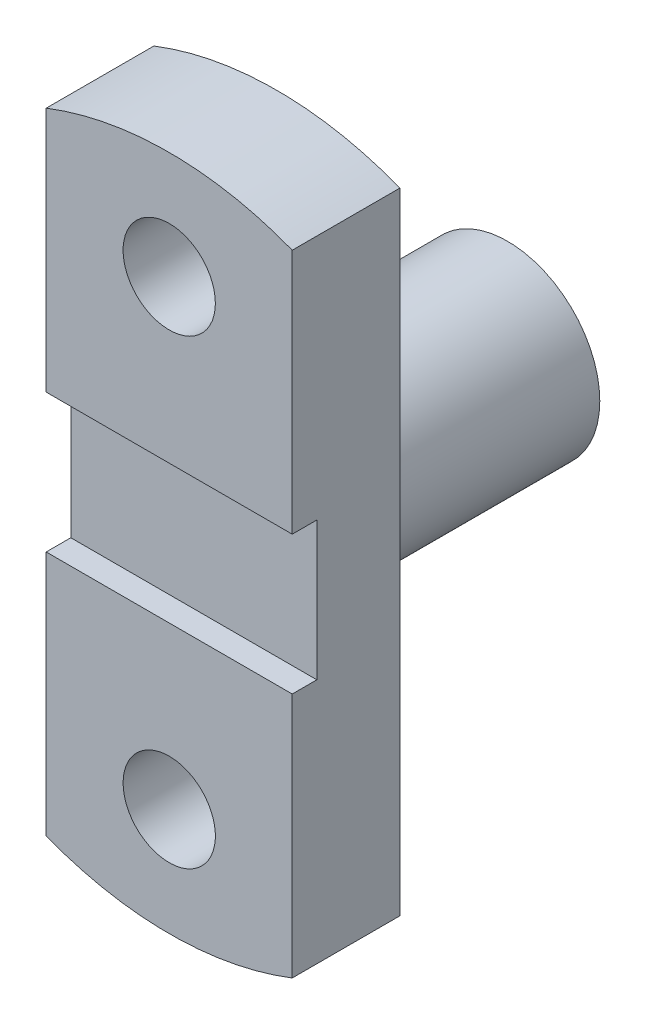
ISO-10303-21;
HEADER;
FILE_DESCRIPTION(('STEP AP214'),'2;1');
FILE_NAME('part.step','',(''),(''),'','','');
FILE_SCHEMA(('AUTOMOTIVE_DESIGN { 1 0 10303 214 1 1 1 1 }'));
ENDSEC;
DATA;
#1=APPLICATION_CONTEXT('core data for automotive mechanical design processes');
#2=APPLICATION_PROTOCOL_DEFINITION('international standard','automotive_design',2000,#1);
#3=PRODUCT_CONTEXT('',#1,'mechanical');
#4=PRODUCT('Part','Part','',(#3));
#5=PRODUCT_RELATED_PRODUCT_CATEGORY('part','',(#4));
#6=PRODUCT_DEFINITION_FORMATION('','',#4);
#7=PRODUCT_DEFINITION_CONTEXT('part definition',#1,'design');
#8=PRODUCT_DEFINITION('design','',#6,#7);
#9=PRODUCT_DEFINITION_SHAPE('','',#8);
#10=(LENGTH_UNIT() NAMED_UNIT(*) SI_UNIT(.MILLI.,.METRE.));
#11=(NAMED_UNIT(*) PLANE_ANGLE_UNIT() SI_UNIT($,.RADIAN.));
#12=(NAMED_UNIT(*) SI_UNIT($,.STERADIAN.) SOLID_ANGLE_UNIT());
#13=UNCERTAINTY_MEASURE_WITH_UNIT(LENGTH_MEASURE(1.E-05),#10,'distance_accuracy_value','');
#14=(GEOMETRIC_REPRESENTATION_CONTEXT(3) GLOBAL_UNCERTAINTY_ASSIGNED_CONTEXT((#13)) GLOBAL_UNIT_ASSIGNED_CONTEXT((#10,
#11,#12)) REPRESENTATION_CONTEXT('',''));
#15=CARTESIAN_POINT('',(0.,0.,0.));
#16=DIRECTION('',(0.,0.,1.));
#17=DIRECTION('',(1.,0.,0.));
#18=AXIS2_PLACEMENT_3D('',#15,#16,#17);
#19=CARTESIAN_POINT('',(0.,0.,17.5));
#20=DIRECTION('',(0.,0.,-1.));
#21=DIRECTION('',(-1.,0.,0.));
#22=AXIS2_PLACEMENT_3D('',#19,#20,#21);
#23=PLANE('',#22);
#24=CARTESIAN_POINT('',(0.,75.,17.5));
#25=DIRECTION('',(0.,0.,1.));
#26=DIRECTION('',(1.,0.,0.));
#27=AXIS2_PLACEMENT_3D('',#24,#25,#26);
#28=CIRCLE('',#27,15.);
#29=CARTESIAN_POINT('',(15.,75.,17.5));
#30=VERTEX_POINT('',#29);
#31=EDGE_CURVE('E153',#30,#30,#28,.T.);
#32=ORIENTED_EDGE('',*,*,#31,.F.);
#33=EDGE_LOOP('',(#32));
#34=FACE_BOUND('',#33,.T.);
#35=DIRECTION('',(0.,-1.,0.));
#36=VECTOR('',#35,1.);
#37=CARTESIAN_POINT('',(-40.,-102.469507659596,17.5));
#38=LINE('',#37,#36);
#39=CARTESIAN_POINT('',(-40.,102.469507659596,17.5));
#40=VERTEX_POINT('',#39);
#41=CARTESIAN_POINT('',(-40.,22.5,17.5));
#42=VERTEX_POINT('',#41);
#43=EDGE_CURVE('E95',#40,#42,#38,.T.);
#44=ORIENTED_EDGE('',*,*,#43,.T.);
#45=DIRECTION('',(1.,0.,0.));
#46=VECTOR('',#45,1.);
#47=CARTESIAN_POINT('',(-85.7055795281058,22.5,17.5));
#48=LINE('',#47,#46);
#49=CARTESIAN_POINT('',(40.,22.5,17.5));
#50=VERTEX_POINT('',#49);
#51=EDGE_CURVE('E136',#42,#50,#48,.T.);
#52=ORIENTED_EDGE('',*,*,#51,.T.);
#53=DIRECTION('',(0.,1.,0.));
#54=VECTOR('',#53,1.);
#55=CARTESIAN_POINT('',(40.,-102.469507659596,17.5));
#56=LINE('',#55,#54);
#57=CARTESIAN_POINT('',(40.,102.469507659596,17.5));
#58=VERTEX_POINT('',#57);
#59=EDGE_CURVE('E62',#50,#58,#56,.T.);
#60=ORIENTED_EDGE('',*,*,#59,.T.);
#61=CARTESIAN_POINT('',(0.,0.,17.5));
#62=DIRECTION('',(0.,0.,1.));
#63=DIRECTION('',(-1.,0.,0.));
#64=AXIS2_PLACEMENT_3D('',#61,#62,#63);
#65=CIRCLE('',#64,110.);
#66=EDGE_CURVE('E157',#58,#40,#65,.T.);
#67=ORIENTED_EDGE('',*,*,#66,.T.);
#68=EDGE_LOOP('',(#44,#52,#60,#67));
#69=FACE_BOUND('',#68,.T.);
#70=ADVANCED_FACE('F39',(#34,#69),#23,.F.);
#71=CARTESIAN_POINT('',(40.,-102.469507659596,17.5));
#72=VERTEX_POINT('',#71);
#73=CARTESIAN_POINT('',(40.,-22.5,17.5));
#74=VERTEX_POINT('',#73);
#75=EDGE_CURVE('E164',#72,#74,#56,.T.);
#76=ORIENTED_EDGE('',*,*,#75,.T.);
#77=DIRECTION('',(1.,0.,0.));
#78=VECTOR('',#77,1.);
#79=CARTESIAN_POINT('',(-85.7055795281058,-22.5,17.5));
#80=LINE('',#79,#78);
#81=CARTESIAN_POINT('',(-40.,-22.5,17.5));
#82=VERTEX_POINT('',#81);
#83=EDGE_CURVE('E53',#82,#74,#80,.T.);
#84=ORIENTED_EDGE('',*,*,#83,.F.);
#85=CARTESIAN_POINT('',(-40.,-102.469507659596,17.5));
#86=VERTEX_POINT('',#85);
#87=EDGE_CURVE('E161',#82,#86,#38,.T.);
#88=ORIENTED_EDGE('',*,*,#87,.T.);
#89=CARTESIAN_POINT('',(0.,0.,17.5));
#90=DIRECTION('',(0.,0.,1.));
#91=DIRECTION('',(1.,0.,0.));
#92=AXIS2_PLACEMENT_3D('',#89,#90,#91);
#93=CIRCLE('',#92,110.);
#94=EDGE_CURVE('E162',#86,#72,#93,.T.);
#95=ORIENTED_EDGE('',*,*,#94,.T.);
#96=EDGE_LOOP('',(#76,#84,#88,#95));
#97=FACE_BOUND('',#96,.T.);
#98=CARTESIAN_POINT('',(0.,-74.9999999999999,17.5));
#99=DIRECTION('',(0.,0.,1.));
#100=DIRECTION('',(-1.,0.,0.));
#101=AXIS2_PLACEMENT_3D('',#98,#99,#100);
#102=CIRCLE('',#101,15.);
#103=CARTESIAN_POINT('',(-15.,-74.9999999999999,17.5));
#104=VERTEX_POINT('',#103);
#105=EDGE_CURVE('E150',#104,#104,#102,.T.);
#106=ORIENTED_EDGE('',*,*,#105,.F.);
#107=EDGE_LOOP('',(#106));
#108=FACE_BOUND('',#107,.T.);
#109=ADVANCED_FACE('F213',(#97,#108),#23,.F.);
#110=CARTESIAN_POINT('',(0.,0.,-17.5));
#111=DIRECTION('',(0.,0.,-1.));
#112=DIRECTION('',(-1.,0.,0.));
#113=AXIS2_PLACEMENT_3D('',#110,#111,#112);
#114=PLANE('',#113);
#115=CARTESIAN_POINT('',(0.,0.,-17.5));
#116=DIRECTION('',(0.,0.,-1.));
#117=DIRECTION('',(-1.,0.,0.));
#118=AXIS2_PLACEMENT_3D('',#115,#116,#117);
#119=CIRCLE('',#118,30.);
#120=CARTESIAN_POINT('',(-30.,0.,-17.5));
#121=VERTEX_POINT('',#120);
#122=EDGE_CURVE('E197',#121,#121,#119,.T.);
#123=ORIENTED_EDGE('',*,*,#122,.F.);
#124=EDGE_LOOP('',(#123));
#125=FACE_BOUND('',#124,.T.);
#126=CARTESIAN_POINT('',(0.,75.,-17.5));
#127=DIRECTION('',(0.,0.,1.));
#128=DIRECTION('',(1.,0.,0.));
#129=AXIS2_PLACEMENT_3D('',#126,#127,#128);
#130=CIRCLE('',#129,15.);
#131=CARTESIAN_POINT('',(15.,75.,-17.5));
#132=VERTEX_POINT('',#131);
#133=EDGE_CURVE('E147',#132,#132,#130,.T.);
#134=ORIENTED_EDGE('',*,*,#133,.T.);
#135=EDGE_LOOP('',(#134));
#136=FACE_BOUND('',#135,.T.);
#137=CARTESIAN_POINT('',(0.,0.,-17.5));
#138=DIRECTION('',(0.,0.,1.));
#139=DIRECTION('',(-1.,0.,0.));
#140=AXIS2_PLACEMENT_3D('',#137,#138,#139);
#141=CIRCLE('',#140,110.);
#142=CARTESIAN_POINT('',(40.,102.469507659596,-17.5));
#143=VERTEX_POINT('',#142);
#144=CARTESIAN_POINT('',(-40.,102.469507659596,-17.5));
#145=VERTEX_POINT('',#144);
#146=EDGE_CURVE('E156',#143,#145,#141,.T.);
#147=ORIENTED_EDGE('',*,*,#146,.F.);
#148=DIRECTION('',(0.,1.,0.));
#149=VECTOR('',#148,1.);
#150=CARTESIAN_POINT('',(40.,-102.469507659596,-17.5));
#151=LINE('',#150,#149);
#152=CARTESIAN_POINT('',(40.,-102.469507659596,-17.5));
#153=VERTEX_POINT('',#152);
#154=EDGE_CURVE('E83',#153,#143,#151,.T.);
#155=ORIENTED_EDGE('',*,*,#154,.F.);
#156=CARTESIAN_POINT('',(0.,0.,-17.5));
#157=DIRECTION('',(0.,0.,1.));
#158=DIRECTION('',(1.,0.,0.));
#159=AXIS2_PLACEMENT_3D('',#156,#157,#158);
#160=CIRCLE('',#159,110.);
#161=CARTESIAN_POINT('',(-40.,-102.469507659596,-17.5));
#162=VERTEX_POINT('',#161);
#163=EDGE_CURVE('E175',#162,#153,#160,.T.);
#164=ORIENTED_EDGE('',*,*,#163,.F.);
#165=DIRECTION('',(0.,-1.,0.));
#166=VECTOR('',#165,1.);
#167=CARTESIAN_POINT('',(-40.,-102.469507659596,-17.5));
#168=LINE('',#167,#166);
#169=EDGE_CURVE('E168',#145,#162,#168,.T.);
#170=ORIENTED_EDGE('',*,*,#169,.F.);
#171=EDGE_LOOP('',(#147,#155,#164,#170));
#172=FACE_BOUND('',#171,.T.);
#173=CARTESIAN_POINT('',(0.,-74.9999999999999,-17.5));
#174=DIRECTION('',(0.,0.,1.));
#175=DIRECTION('',(-1.,0.,0.));
#176=AXIS2_PLACEMENT_3D('',#173,#174,#175);
#177=CIRCLE('',#176,15.);
#178=CARTESIAN_POINT('',(-15.,-74.9999999999999,-17.5));
#179=VERTEX_POINT('',#178);
#180=EDGE_CURVE('E144',#179,#179,#177,.T.);
#181=ORIENTED_EDGE('',*,*,#180,.T.);
#182=EDGE_LOOP('',(#181));
#183=FACE_BOUND('',#182,.T.);
#184=ADVANCED_FACE('F190',(#125,#136,#172,#183),#114,.T.);
#185=CARTESIAN_POINT('',(0.,0.,17.5));
#186=DIRECTION('',(0.,0.,-1.));
#187=DIRECTION('',(-1.,0.,0.));
#188=AXIS2_PLACEMENT_3D('',#185,#186,#187);
#189=CYLINDRICAL_SURFACE('',#188,110.);
#190=ORIENTED_EDGE('',*,*,#146,.T.);
#191=DIRECTION('',(0.,0.,-1.));
#192=VECTOR('',#191,1.);
#193=CARTESIAN_POINT('',(-40.,102.469507659596,17.5));
#194=LINE('',#193,#192);
#195=EDGE_CURVE('E11',#40,#145,#194,.T.);
#196=ORIENTED_EDGE('',*,*,#195,.F.);
#197=ORIENTED_EDGE('',*,*,#66,.F.);
#198=DIRECTION('',(0.,0.,-1.));
#199=VECTOR('',#198,1.);
#200=CARTESIAN_POINT('',(40.,102.469507659596,17.5));
#201=LINE('',#200,#199);
#202=EDGE_CURVE('E170',#58,#143,#201,.T.);
#203=ORIENTED_EDGE('',*,*,#202,.T.);
#204=EDGE_LOOP('',(#190,#196,#197,#203));
#205=FACE_BOUND('',#204,.T.);
#206=ADVANCED_FACE('F41',(#205),#189,.T.);
#207=CARTESIAN_POINT('',(-40.,-102.469507659596,17.5));
#208=DIRECTION('',(1.,0.,0.));
#209=DIRECTION('',(0.,0.,-1.));
#210=AXIS2_PLACEMENT_3D('',#207,#208,#209);
#211=PLANE('',#210);
#212=DIRECTION('',(0.,-1.,0.));
#213=VECTOR('',#212,1.);
#214=CARTESIAN_POINT('',(-40.,22.5,9.5));
#215=LINE('',#214,#213);
#216=CARTESIAN_POINT('',(-40.,22.5,9.5));
#217=VERTEX_POINT('',#216);
#218=CARTESIAN_POINT('',(-40.,-22.5,9.5));
#219=VERTEX_POINT('',#218);
#220=EDGE_CURVE('E124',#217,#219,#215,.T.);
#221=ORIENTED_EDGE('',*,*,#220,.F.);
#222=DIRECTION('',(0.,0.,-1.));
#223=VECTOR('',#222,1.);
#224=CARTESIAN_POINT('',(-40.,22.5,17.5));
#225=LINE('',#224,#223);
#226=EDGE_CURVE('E148',#42,#217,#225,.T.);
#227=ORIENTED_EDGE('',*,*,#226,.F.);
#228=ORIENTED_EDGE('',*,*,#43,.F.);
#229=ORIENTED_EDGE('',*,*,#195,.T.);
#230=ORIENTED_EDGE('',*,*,#169,.T.);
#231=DIRECTION('',(0.,0.,-1.));
#232=VECTOR('',#231,1.);
#233=CARTESIAN_POINT('',(-40.,-102.469507659596,17.5));
#234=LINE('',#233,#232);
#235=EDGE_CURVE('E50',#86,#162,#234,.T.);
#236=ORIENTED_EDGE('',*,*,#235,.F.);
#237=ORIENTED_EDGE('',*,*,#87,.F.);
#238=DIRECTION('',(0.,0.,1.));
#239=VECTOR('',#238,1.);
#240=CARTESIAN_POINT('',(-40.,-22.5,9.5));
#241=LINE('',#240,#239);
#242=EDGE_CURVE('E141',#219,#82,#241,.T.);
#243=ORIENTED_EDGE('',*,*,#242,.F.);
#244=EDGE_LOOP('',(#221,#227,#228,#229,#230,#236,#237,#243));
#245=FACE_BOUND('',#244,.T.);
#246=ADVANCED_FACE('F191',(#245),#211,.F.);
#247=CARTESIAN_POINT('',(0.,0.,17.5));
#248=DIRECTION('',(0.,0.,-1.));
#249=DIRECTION('',(-1.,0.,0.));
#250=AXIS2_PLACEMENT_3D('',#247,#248,#249);
#251=CYLINDRICAL_SURFACE('',#250,110.);
#252=ORIENTED_EDGE('',*,*,#163,.T.);
#253=DIRECTION('',(0.,0.,-1.));
#254=VECTOR('',#253,1.);
#255=CARTESIAN_POINT('',(40.,-102.469507659596,17.5));
#256=LINE('',#255,#254);
#257=EDGE_CURVE('E177',#72,#153,#256,.T.);
#258=ORIENTED_EDGE('',*,*,#257,.F.);
#259=ORIENTED_EDGE('',*,*,#94,.F.);
#260=ORIENTED_EDGE('',*,*,#235,.T.);
#261=EDGE_LOOP('',(#252,#258,#259,#260));
#262=FACE_BOUND('',#261,.T.);
#263=ADVANCED_FACE('F185',(#262),#251,.T.);
#264=CARTESIAN_POINT('',(40.,-102.469507659596,17.5));
#265=DIRECTION('',(-1.,0.,0.));
#266=DIRECTION('',(0.,0.,1.));
#267=AXIS2_PLACEMENT_3D('',#264,#265,#266);
#268=PLANE('',#267);
#269=ORIENTED_EDGE('',*,*,#59,.F.);
#270=DIRECTION('',(0.,0.,1.));
#271=VECTOR('',#270,1.);
#272=CARTESIAN_POINT('',(40.,22.5,17.5));
#273=LINE('',#272,#271);
#274=CARTESIAN_POINT('',(40.,22.5,9.5));
#275=VERTEX_POINT('',#274);
#276=EDGE_CURVE('E133',#275,#50,#273,.T.);
#277=ORIENTED_EDGE('',*,*,#276,.F.);
#278=DIRECTION('',(0.,1.,0.));
#279=VECTOR('',#278,1.);
#280=CARTESIAN_POINT('',(40.,22.5,9.5));
#281=LINE('',#280,#279);
#282=CARTESIAN_POINT('',(40.,-22.5,9.5));
#283=VERTEX_POINT('',#282);
#284=EDGE_CURVE('E119',#283,#275,#281,.T.);
#285=ORIENTED_EDGE('',*,*,#284,.F.);
#286=DIRECTION('',(0.,0.,-1.));
#287=VECTOR('',#286,1.);
#288=CARTESIAN_POINT('',(40.,-22.5,9.5));
#289=LINE('',#288,#287);
#290=EDGE_CURVE('E130',#74,#283,#289,.T.);
#291=ORIENTED_EDGE('',*,*,#290,.F.);
#292=ORIENTED_EDGE('',*,*,#75,.F.);
#293=ORIENTED_EDGE('',*,*,#257,.T.);
#294=ORIENTED_EDGE('',*,*,#154,.T.);
#295=ORIENTED_EDGE('',*,*,#202,.F.);
#296=EDGE_LOOP('',(#269,#277,#285,#291,#292,#293,#294,#295));
#297=FACE_BOUND('',#296,.T.);
#298=ADVANCED_FACE('F132',(#297),#268,.F.);
#299=CARTESIAN_POINT('',(0.,75.,17.5));
#300=DIRECTION('',(0.,0.,-1.));
#301=DIRECTION('',(-1.,0.,0.));
#302=AXIS2_PLACEMENT_3D('',#299,#300,#301);
#303=CYLINDRICAL_SURFACE('',#302,15.);
#304=ORIENTED_EDGE('',*,*,#31,.T.);
#305=EDGE_LOOP('',(#304));
#306=FACE_BOUND('',#305,.T.);
#307=ORIENTED_EDGE('',*,*,#133,.F.);
#308=EDGE_LOOP('',(#307));
#309=FACE_BOUND('',#308,.T.);
#310=ADVANCED_FACE('F220',(#306,#309),#303,.F.);
#311=CARTESIAN_POINT('',(0.,-74.9999999999999,17.5));
#312=DIRECTION('',(0.,0.,-1.));
#313=DIRECTION('',(-1.,0.,0.));
#314=AXIS2_PLACEMENT_3D('',#311,#312,#313);
#315=CYLINDRICAL_SURFACE('',#314,15.);
#316=ORIENTED_EDGE('',*,*,#105,.T.);
#317=EDGE_LOOP('',(#316));
#318=FACE_BOUND('',#317,.T.);
#319=ORIENTED_EDGE('',*,*,#180,.F.);
#320=EDGE_LOOP('',(#319));
#321=FACE_BOUND('',#320,.T.);
#322=ADVANCED_FACE('F218',(#318,#321),#315,.F.);
#323=CARTESIAN_POINT('',(-85.7055795281058,22.5,17.5));
#324=DIRECTION('',(0.,1.,0.));
#325=DIRECTION('',(0.,0.,1.));
#326=AXIS2_PLACEMENT_3D('',#323,#324,#325);
#327=PLANE('',#326);
#328=ORIENTED_EDGE('',*,*,#226,.T.);
#329=DIRECTION('',(1.,0.,0.));
#330=VECTOR('',#329,1.);
#331=CARTESIAN_POINT('',(-85.7055795281058,22.5,9.5));
#332=LINE('',#331,#330);
#333=EDGE_CURVE('E123',#217,#275,#332,.T.);
#334=ORIENTED_EDGE('',*,*,#333,.T.);
#335=ORIENTED_EDGE('',*,*,#276,.T.);
#336=ORIENTED_EDGE('',*,*,#51,.F.);
#337=EDGE_LOOP('',(#328,#334,#335,#336));
#338=FACE_BOUND('',#337,.T.);
#339=ADVANCED_FACE('F194',(#338),#327,.F.);
#340=CARTESIAN_POINT('',(-85.7055795281058,22.5,9.5));
#341=DIRECTION('',(0.,0.,-1.));
#342=DIRECTION('',(-1.,0.,0.));
#343=AXIS2_PLACEMENT_3D('',#340,#341,#342);
#344=PLANE('',#343);
#345=ORIENTED_EDGE('',*,*,#220,.T.);
#346=DIRECTION('',(1.,0.,0.));
#347=VECTOR('',#346,1.);
#348=CARTESIAN_POINT('',(-85.7055795281058,-22.5,9.5));
#349=LINE('',#348,#347);
#350=EDGE_CURVE('E116',#219,#283,#349,.T.);
#351=ORIENTED_EDGE('',*,*,#350,.T.);
#352=ORIENTED_EDGE('',*,*,#284,.T.);
#353=ORIENTED_EDGE('',*,*,#333,.F.);
#354=EDGE_LOOP('',(#345,#351,#352,#353));
#355=FACE_BOUND('',#354,.T.);
#356=ADVANCED_FACE('F120',(#355),#344,.F.);
#357=CARTESIAN_POINT('',(-85.7055795281058,-22.5,9.5));
#358=DIRECTION('',(0.,-1.,0.));
#359=DIRECTION('',(0.,0.,-1.));
#360=AXIS2_PLACEMENT_3D('',#357,#358,#359);
#361=PLANE('',#360);
#362=ORIENTED_EDGE('',*,*,#242,.T.);
#363=ORIENTED_EDGE('',*,*,#83,.T.);
#364=ORIENTED_EDGE('',*,*,#290,.T.);
#365=ORIENTED_EDGE('',*,*,#350,.F.);
#366=EDGE_LOOP('',(#362,#363,#364,#365));
#367=FACE_BOUND('',#366,.T.);
#368=ADVANCED_FACE('F126',(#367),#361,.F.);
#369=CARTESIAN_POINT('',(0.,0.,-92.5));
#370=DIRECTION('',(0.,0.,1.));
#371=DIRECTION('',(1.,0.,0.));
#372=AXIS2_PLACEMENT_3D('',#369,#370,#371);
#373=CYLINDRICAL_SURFACE('',#372,30.);
#374=CARTESIAN_POINT('',(0.,0.,-92.5));
#375=DIRECTION('',(0.,0.,-1.));
#376=DIRECTION('',(-1.,0.,0.));
#377=AXIS2_PLACEMENT_3D('',#374,#375,#376);
#378=CIRCLE('',#377,30.);
#379=CARTESIAN_POINT('',(-30.,0.,-92.5));
#380=VERTEX_POINT('',#379);
#381=EDGE_CURVE('E131',#380,#380,#378,.T.);
#382=ORIENTED_EDGE('',*,*,#381,.F.);
#383=EDGE_LOOP('',(#382));
#384=FACE_BOUND('',#383,.T.);
#385=ORIENTED_EDGE('',*,*,#122,.T.);
#386=EDGE_LOOP('',(#385));
#387=FACE_BOUND('',#386,.T.);
#388=ADVANCED_FACE('F202',(#384,#387),#373,.T.);
#389=CARTESIAN_POINT('',(0.,0.,-92.5));
#390=DIRECTION('',(0.,0.,-1.));
#391=DIRECTION('',(-1.,0.,0.));
#392=AXIS2_PLACEMENT_3D('',#389,#390,#391);
#393=PLANE('',#392);
#394=ORIENTED_EDGE('',*,*,#381,.T.);
#395=EDGE_LOOP('',(#394));
#396=FACE_BOUND('',#395,.T.);
#397=ADVANCED_FACE('F201',(#396),#393,.T.);
#398=CLOSED_SHELL('',(#70,#109,#184,#206,#246,#263,#298,#310,#322,#339,#356,#368,#388,#397));
#399=MANIFOLD_SOLID_BREP('B2',#398);
#400=ADVANCED_BREP_SHAPE_REPRESENTATION('',(#18,#399),#14);
#401=SHAPE_DEFINITION_REPRESENTATION(#9,#400);
ENDSEC;
END-ISO-10303-21;
